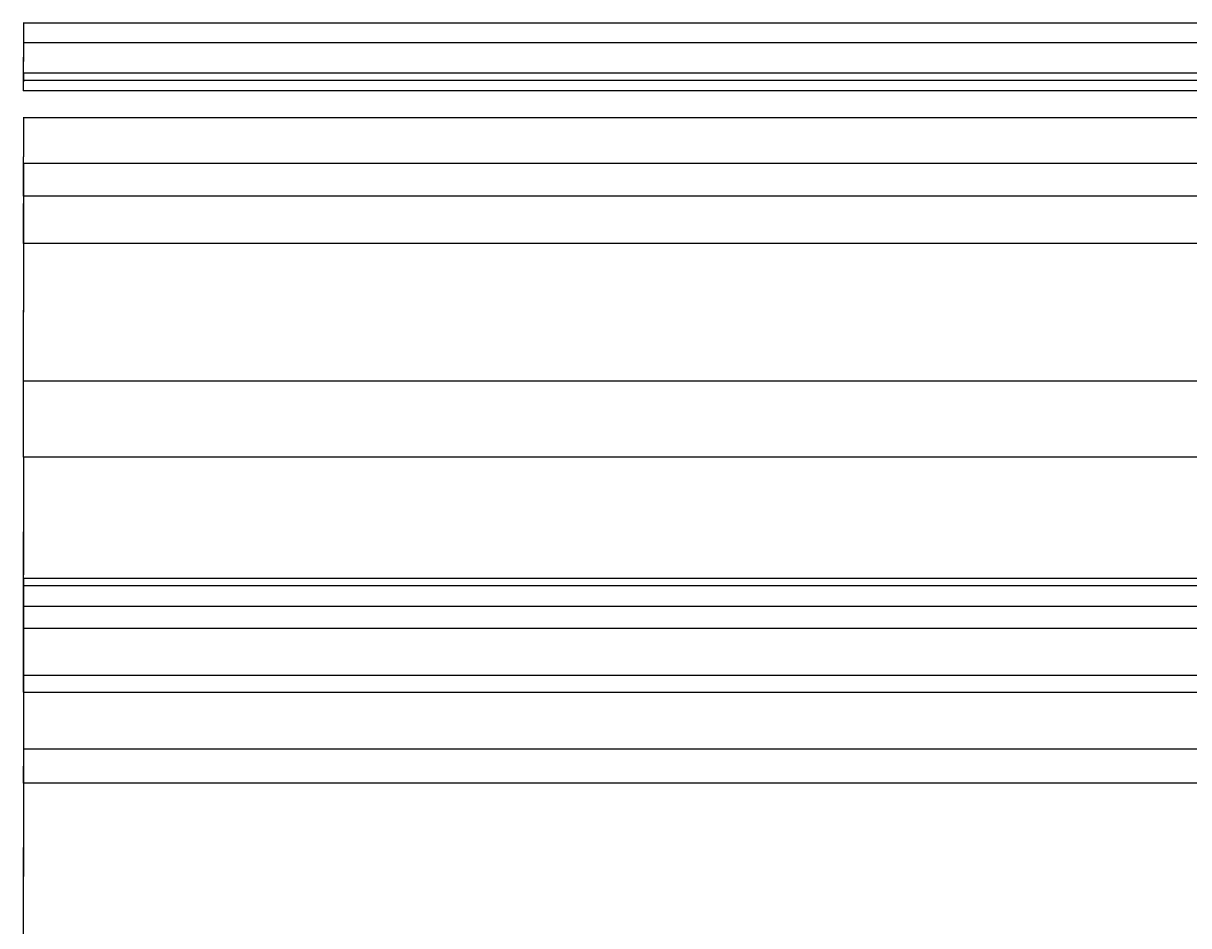
# Model space of a CAD drawing. Units: inches. Extents: x 35362 to 73946, y 43607 to 67532.
# Tile 129 of 134: x 35362 to 46600, y 56772 to 65479. Entities that reach past the tile are written whole.
import ezdxf

# ---------------------------------------------------------------- set-up
doc = ezdxf.new("R2010")
doc.units = ezdxf.units.IN
doc.header["$MEASUREMENT"] = 0
doc.layers.add('A-ANNO-DIMS', color=2, linetype='Continuous', lineweight=18)
doc.styles.get("Standard").update_dxf_attribs({"font": 'arial.ttf'})
doc.dimstyles.get("Standard").update_dxf_attribs({"dimtxt": 0.18, "dimasz": 0.18, "dimexe": 0.18, "dimexo": 0.0625, "dimgap": 0.09, "dimtad": 0, "dimtih": 1, "dimtoh": 1, "dimdec": 4, "dimzin": 0, "dimdsep": 46, "dimtxsty": 'Standard', "dimcen": 0.09, "dimadec": 0, "dimazin": 0, "dimtfac": 1, "dimtdec": 4, "dimtofl": 0, "dimtmove": 0, "dimatfit": 3, "dimfxl": 1, "dimtolj": 1, "dimtzin": 0, "dimarcsym": 0})

# ---------------------------------------------------------------- blocks, each defined once
blk = doc.blocks.new('*D12')
at = {"layer": 'A-ANNO-DIMS', "color": 0, "lineweight": -2, "transparency": 16777216}
for p, q in [((47978.60234600001, 59023.27631300003), (35361.76908500003, 59023.27631300003)), ((35361.94908500003, 59023.09631300003), (35361.94908500003, 57526.23819563782)), ((35361.94908500003, 56029.01627200003), (35361.94908500003, 57525.87438936224)), ((47978.60234600001, 56028.83627200003), (35361.76908500003, 56028.83627200003))]:
    blk.add_line(p, q, dxfattribs=at)
at = {"layer": 'A-ANNO-DIMS', "color": 0, "transparency": 16777216}
for points in [[(35361.91908500003, 59023.09631300003), (35361.97908500003, 59023.09631300003), (35361.94908500003, 59023.27631300003)], [(35361.91908500003, 56029.01627200003), (35361.97908500003, 56029.01627200003), (35361.94908500003, 56028.83627200003)]]:
    blk.add_solid(points, dxfattribs=at)
at = {"layer": 'Defpoints', "color": 0, "transparency": 16777216}
for p in [(47978.66484600001, 59023.27631300003), (35361.94908500003, 56028.83627200003), (47978.66484600001, 56028.83627200003)]:
    blk.add_point(p, dxfattribs=at)
at = {"layer": 'A-ANNO-DIMS', "color": 0, "transparency": 16777216, "insert": (35361.94908500004, 57526.05629250001), "char_height": 0.18, "attachment_point": 5}
blk.add_mtext('\\A1;2994.4', dxfattribs=at)
blk = doc.blocks.new('*D18')
at = {"layer": 'A-ANNO-DIMS', "color": 0, "lineweight": -2, "transparency": 16777216}
for p, q in [((49923.24483100003, 64127.44160800003), (35361.76908500003, 64127.44160800002)), ((35361.94908500003, 64127.26160800002), (35361.94908500003, 62710.54579452935)), ((35361.94908500003, 61293.46605200002), (35361.94908500003, 62710.18186547069)), ((49923.24483100003, 61293.28605200003), (35361.76908500003, 61293.28605200003))]:
    blk.add_line(p, q, dxfattribs=at)
at = {"layer": 'A-ANNO-DIMS', "color": 0, "transparency": 16777216}
for points in [[(35361.91908500003, 64127.26160800002), (35361.97908500003, 64127.26160800002), (35361.94908500003, 64127.44160800002)], [(35361.91908500003, 61293.46605200002), (35361.97908500003, 61293.46605200002), (35361.94908500003, 61293.28605200003)]]:
    blk.add_solid(points, dxfattribs=at)
at = {"layer": 'Defpoints', "color": 0, "transparency": 16777216}
for p in [(49923.30733100003, 64127.44160800003), (35361.94908500003, 61293.28605200003), (49923.30733100003, 61293.28605200003)]:
    blk.add_point(p, dxfattribs=at)
at = {"layer": 'A-ANNO-DIMS', "color": 0, "transparency": 16777216, "insert": (35361.94908500005, 62710.36383), "char_height": 0.18, "attachment_point": 5}
blk.add_mtext('\\A1;2834', dxfattribs=at)
blk = doc.blocks.new('*D28')
at = {"layer": 'A-ANNO-DIMS', "color": 0, "lineweight": -2, "transparency": 16777216}
for p, q in [((49923.24483100003, 61293.28605200003), (35361.76908500003, 61293.28605200003)), ((35361.94908500003, 61293.10605200002), (35361.94908500003, 60158.46308563782)), ((35361.94908500003, 59023.45631300003), (35361.94908500003, 60158.09927936224)), ((47978.60234600001, 59023.27631300003), (35361.76908500003, 59023.27631300003))]:
    blk.add_line(p, q, dxfattribs=at)
at = {"layer": 'A-ANNO-DIMS', "color": 0, "transparency": 16777216}
for points in [[(35361.91908500003, 61293.10605200002), (35361.97908500003, 61293.10605200002), (35361.94908500003, 61293.28605200003)], [(35361.91908500003, 59023.45631300003), (35361.97908500003, 59023.45631300003), (35361.94908500003, 59023.27631300003)]]:
    blk.add_solid(points, dxfattribs=at)
at = {"layer": 'Defpoints', "color": 0, "transparency": 16777216}
for p in [(49923.30733100003, 61293.28605200003), (35361.94908500003, 59023.27631300003), (47978.66484600001, 59023.27631300003)]:
    blk.add_point(p, dxfattribs=at)
at = {"layer": 'A-ANNO-DIMS', "color": 0, "transparency": 16777216, "insert": (35361.94908500005, 60158.2811825), "char_height": 0.18, "attachment_point": 5}
blk.add_mtext('\\A1;2270.0', dxfattribs=at)
blk = doc.blocks.new('*D34')
at = {"layer": 'A-ANNO-DIMS', "color": 0, "lineweight": -2, "transparency": 16777216}
for p, q in [((65335.95350800003, 61293.28605200003), (35361.76908500003, 61293.28605200003)), ((35361.94908500003, 61293.10605200002), (35361.94908500003, 60239.39690763781)), ((35361.94908500003, 59185.32395700002), (35361.94908500003, 60239.03310136224)), ((61240.84483600002, 59185.14395700003), (35361.76908500003, 59185.14395700002))]:
    blk.add_line(p, q, dxfattribs=at)
at = {"layer": 'A-ANNO-DIMS', "color": 0, "transparency": 16777216}
for points in [[(35361.91908500003, 61293.10605200002), (35361.97908500003, 61293.10605200002), (35361.94908500003, 61293.28605200003)], [(35361.91908500003, 59185.32395700002), (35361.97908500003, 59185.32395700002), (35361.94908500003, 59185.14395700002)]]:
    blk.add_solid(points, dxfattribs=at)
at = {"layer": 'Defpoints', "color": 0, "transparency": 16777216}
for p in [(65336.01600800003, 61293.28605200003), (35361.94908500003, 59185.14395700002), (61240.90733600002, 59185.14395700003)]:
    blk.add_point(p, dxfattribs=at)
at = {"layer": 'A-ANNO-DIMS', "color": 0, "transparency": 16777216, "insert": (35361.94908500005, 60239.2150045), "char_height": 0.18, "attachment_point": 5}
blk.add_mtext('\\A1;2108.1', dxfattribs=at)
blk = doc.blocks.new('*D36')
at = {"layer": 'A-ANNO-DIMS', "color": 0, "lineweight": -2, "transparency": 16777216}
for p, q in [((68320.80826200004, 60122.34633200002), (35361.76908500003, 60122.34633200002)), ((35361.94908500003, 60122.16633200002), (35361.94908500003, 57247.82893113781)), ((35361.94908500003, 54373.12772400002), (35361.94908500003, 57247.46512486223)), ((68320.80826200004, 54372.94772400003), (35361.76908500003, 54372.94772400002))]:
    blk.add_line(p, q, dxfattribs=at)
at = {"layer": 'A-ANNO-DIMS', "color": 0, "transparency": 16777216}
for points in [[(35361.91908500003, 60122.16633200002), (35361.97908500003, 60122.16633200002), (35361.94908500003, 60122.34633200002)], [(35361.91908500003, 54373.12772400002), (35361.97908500003, 54373.12772400002), (35361.94908500003, 54372.94772400002)]]:
    blk.add_solid(points, dxfattribs=at)
at = {"layer": 'Defpoints', "color": 0, "transparency": 16777216}
for p in [(68320.87076200004, 60122.34633200002), (35361.94908500003, 54372.94772400002), (68320.87076200004, 54372.94772400003)]:
    blk.add_point(p, dxfattribs=at)
at = {"layer": 'A-ANNO-DIMS', "color": 0, "transparency": 16777216, "insert": (35361.94908500004, 57247.64702799999), "char_height": 0.18, "attachment_point": 5}
blk.add_mtext('\\A1;5749.4', dxfattribs=at)
blk = doc.blocks.new('*D45')
at = {"layer": 'A-ANNO-DIMS', "color": 0, "lineweight": -2, "transparency": 16777216}
for p, q in [((52517.73527400002, 65478.87035600003), (35361.76908500003, 65478.87035600002)), ((35361.94908500003, 65478.69035600002), (35361.94908500003, 65153.89527602935)), ((35361.94908500003, 64828.73626700002), (35361.94908500003, 65153.53134697069)), ((52517.73527400002, 64828.55626700002), (35361.76908500003, 64828.55626700002))]:
    blk.add_line(p, q, dxfattribs=at)
at = {"layer": 'A-ANNO-DIMS', "color": 0, "transparency": 16777216}
for points in [[(35361.91908500003, 65478.69035600002), (35361.97908500003, 65478.69035600002), (35361.94908500003, 65478.87035600002)], [(35361.91908500003, 64828.73626700002), (35361.97908500003, 64828.73626700002), (35361.94908500003, 64828.55626700002)]]:
    blk.add_solid(points, dxfattribs=at)
at = {"layer": 'Defpoints', "color": 0, "transparency": 16777216}
for p in [(52517.79777400003, 65478.87035600003), (35361.94908500003, 64828.55626700002), (52517.79777400003, 64828.55626700002)]:
    blk.add_point(p, dxfattribs=at)
at = {"layer": 'A-ANNO-DIMS', "color": 0, "transparency": 16777216, "insert": (35361.94908500005, 65153.7133115), "char_height": 0.18, "attachment_point": 5}
blk.add_mtext('\\A1;650.3', dxfattribs=at)
blk = doc.blocks.new('*D48')
at = {"layer": 'A-ANNO-DIMS', "color": 0, "lineweight": -2, "transparency": 16777216}
for p, q in [((56457.22713600003, 58474.86812300003), (35361.76908500003, 58474.86812300002)), ((35361.94908500003, 58474.68812300002), (35361.94908500003, 58311.09546902935)), ((35361.94908500003, 58147.13888600002), (35361.94908500003, 58310.73153997069)), ((56457.22713600003, 58146.95888600002), (35361.76908500003, 58146.95888600002))]:
    blk.add_line(p, q, dxfattribs=at)
at = {"layer": 'A-ANNO-DIMS', "color": 0, "transparency": 16777216}
for points in [[(35361.91908500003, 58474.68812300002), (35361.97908500003, 58474.68812300002), (35361.94908500003, 58474.86812300002)], [(35361.91908500003, 58147.13888600002), (35361.97908500003, 58147.13888600002), (35361.94908500003, 58146.95888600002)]]:
    blk.add_solid(points, dxfattribs=at)
at = {"layer": 'Defpoints', "color": 0, "transparency": 16777216}
for p in [(56457.28963600003, 58474.86812300003), (35361.94908500003, 58146.95888600002), (56457.28963600003, 58146.95888600002)]:
    blk.add_point(p, dxfattribs=at)
at = {"layer": 'A-ANNO-DIMS', "color": 0, "transparency": 16777216, "insert": (35361.94908500004, 58310.9135045), "char_height": 0.18, "attachment_point": 5}
blk.add_mtext('\\A1;327.9', dxfattribs=at)
blk = doc.blocks.new('*D73')
at = {"layer": 'A-ANNO-DIMS', "color": 0, "lineweight": -2, "transparency": 16777216}
for p, q in [((59468.73309100003, 64567.97198600003), (35361.76908500003, 64567.97198600002)), ((35361.94908500003, 64567.79198600002), (35361.94908500003, 64189.84474213781)), ((35361.94908500003, 63811.53369200002), (35361.94908500003, 64189.48093586223)), ((59468.73309100003, 63811.35369200002), (35361.76908500003, 63811.35369200002))]:
    blk.add_line(p, q, dxfattribs=at)
at = {"layer": 'A-ANNO-DIMS', "color": 0, "transparency": 16777216}
for points in [[(35361.91908500003, 64567.79198600002), (35361.97908500003, 64567.79198600002), (35361.94908500003, 64567.97198600002)], [(35361.91908500003, 63811.53369200002), (35361.97908500003, 63811.53369200002), (35361.94908500003, 63811.35369200002)]]:
    blk.add_solid(points, dxfattribs=at)
at = {"layer": 'Defpoints', "color": 0, "transparency": 16777216}
for p in [(35361.94908500003, 64567.97198600002), (59468.79559100003, 64567.97198600003), (59468.79559100003, 63811.35369200002)]:
    blk.add_point(p, dxfattribs=at)
at = {"layer": 'A-ANNO-DIMS', "color": 0, "transparency": 16777216, "insert": (35361.94908500005, 64189.66283899999), "char_height": 0.18, "attachment_point": 5}
blk.add_mtext('\\A1;756.6', dxfattribs=at)
blk = doc.blocks.new('*D93')
at = {"layer": 'A-ANNO-DIMS', "color": 0, "lineweight": -2, "transparency": 16777216}
for p, q in [((50377.69713900003, 63354.17630000002), (35361.76908500003, 63354.17630000002)), ((35361.94908500003, 63353.99630000002), (35361.94908500003, 62690.28238902935)), ((35361.94908500003, 62026.20454900002), (35361.94908500003, 62689.91845997069)), ((50377.69713900003, 62026.02454900003), (35361.76908500003, 62026.02454900002))]:
    blk.add_line(p, q, dxfattribs=at)
at = {"layer": 'A-ANNO-DIMS', "color": 0, "transparency": 16777216}
for points in [[(35361.91908500003, 63353.99630000002), (35361.97908500003, 63353.99630000002), (35361.94908500003, 63354.17630000002)], [(35361.91908500003, 62026.20454900002), (35361.97908500003, 62026.20454900002), (35361.94908500003, 62026.02454900002)]]:
    blk.add_solid(points, dxfattribs=at)
at = {"layer": 'Defpoints', "color": 0, "transparency": 16777216}
for p in [(50377.75963900003, 63354.17630000002), (35361.94908500003, 62026.02454900002), (50377.75963900003, 62026.02454900003)]:
    blk.add_point(p, dxfattribs=at)
at = {"layer": 'A-ANNO-DIMS', "color": 0, "transparency": 16777216, "insert": (35361.94908500005, 62690.1004245), "char_height": 0.18, "attachment_point": 5}
blk.add_mtext('\\A1;1328.2', dxfattribs=at)
blk = doc.blocks.new('*D95')
at = {"layer": 'A-ANNO-DIMS', "color": 0, "lineweight": -2, "transparency": 16777216}
for p, q in [((49923.24483100003, 64127.44160800003), (35361.76908500003, 64127.44160800002)), ((35361.94908500003, 64127.26160800002), (35361.94908500003, 63740.99091852935)), ((35361.94908500003, 63354.35630000002), (35361.94908500003, 63740.62698947069)), ((50377.69713900003, 63354.17630000002), (35361.76908500003, 63354.17630000002))]:
    blk.add_line(p, q, dxfattribs=at)
at = {"layer": 'A-ANNO-DIMS', "color": 0, "transparency": 16777216}
for points in [[(35361.91908500003, 64127.26160800002), (35361.97908500003, 64127.26160800002), (35361.94908500003, 64127.44160800002)], [(35361.91908500003, 63354.35630000002), (35361.97908500003, 63354.35630000002), (35361.94908500003, 63354.17630000002)]]:
    blk.add_solid(points, dxfattribs=at)
at = {"layer": 'Defpoints', "color": 0, "transparency": 16777216}
for p in [(49923.30733100003, 64127.44160800003), (35361.94908500003, 63354.17630000002), (50377.75963900003, 63354.17630000002)]:
    blk.add_point(p, dxfattribs=at)
at = {"layer": 'A-ANNO-DIMS', "color": 0, "transparency": 16777216, "insert": (35361.94908500005, 63740.808954), "char_height": 0.18, "attachment_point": 5}
blk.add_mtext('\\A1;773.3', dxfattribs=at)
blk = doc.blocks.new('*D98')
at = {"layer": 'A-ANNO-DIMS', "color": 0, "lineweight": -2, "transparency": 16777216}
for p, q in [((53366.70323300003, 64997.68268100003), (35361.76908500003, 64997.68268100002)), ((35361.94908500003, 64997.50268100002), (35361.94908500003, 64913.30143852935)), ((35361.94908500003, 64828.73626700002), (35361.94908500003, 64912.93750947069)), ((52517.73527400002, 64828.55626700002), (35361.76908500003, 64828.55626700002))]:
    blk.add_line(p, q, dxfattribs=at)
at = {"layer": 'A-ANNO-DIMS', "color": 0, "transparency": 16777216}
for points in [[(35361.91908500003, 64997.50268100002), (35361.97908500003, 64997.50268100002), (35361.94908500003, 64997.68268100002)], [(35361.91908500003, 64828.73626700002), (35361.97908500003, 64828.73626700002), (35361.94908500003, 64828.55626700002)]]:
    blk.add_solid(points, dxfattribs=at)
at = {"layer": 'Defpoints', "color": 0, "transparency": 16777216}
for p in [(53366.76573300002, 64997.68268100003), (35361.94908500003, 64828.55626700002), (52517.79777400003, 64828.55626700002)]:
    blk.add_point(p, dxfattribs=at)
at = {"layer": 'A-ANNO-DIMS', "color": 0, "transparency": 16777216, "insert": (35361.94908500005, 64913.11947399999), "char_height": 0.18, "attachment_point": 5}
blk.add_mtext('\\A1;169.13', dxfattribs=at)
blk = doc.blocks.new('*D101')
at = {"layer": 'A-ANNO-DIMS', "color": 0, "lineweight": -2, "transparency": 16777216}
for p, q in [((52897.41774600003, 65291.58881700003), (35361.76908500003, 65291.58881700002)), ((35361.94908500003, 65291.40881700002), (35361.94908500003, 65109.04535402935)), ((35361.94908500003, 64926.31796200002), (35361.94908500003, 65108.68142497069)), ((53150.59930100002, 64926.13796200003), (35361.76908500003, 64926.13796200002))]:
    blk.add_line(p, q, dxfattribs=at)
at = {"layer": 'A-ANNO-DIMS', "color": 0, "transparency": 16777216}
for points in [[(35361.91908500003, 65291.40881700002), (35361.97908500003, 65291.40881700002), (35361.94908500003, 65291.58881700002)], [(35361.91908500003, 64926.31796200002), (35361.97908500003, 64926.31796200002), (35361.94908500003, 64926.13796200002)]]:
    blk.add_solid(points, dxfattribs=at)
at = {"layer": 'Defpoints', "color": 0, "transparency": 16777216}
for p in [(52897.48024600003, 65291.58881700003), (35361.94908500003, 64926.13796200002), (53150.66180100003, 64926.13796200003)]:
    blk.add_point(p, dxfattribs=at)
at = {"layer": 'A-ANNO-DIMS', "color": 0, "transparency": 16777216, "insert": (35361.94908500005, 65108.8633895), "char_height": 0.18, "attachment_point": 5}
blk.add_mtext('\\A1;365.45', dxfattribs=at)
blk = doc.blocks.new('*D108')
at = {"layer": 'A-ANNO-DIMS', "color": 0, "lineweight": -2, "transparency": 16777216}
for p, q in [((50259.66194000003, 60051.66084400003), (35361.76908500003, 60051.66084400002)), ((35361.94908500003, 60051.48084400002), (35361.94908500003, 59845.07863052935)), ((35361.94908500003, 59638.31248800002), (35361.94908500003, 59844.71470147069)), ((50483.03225800003, 59638.13248800003), (35361.76908500003, 59638.13248800002))]:
    blk.add_line(p, q, dxfattribs=at)
at = {"layer": 'A-ANNO-DIMS', "color": 0, "transparency": 16777216}
for points in [[(35361.91908500003, 60051.48084400002), (35361.97908500003, 60051.48084400002), (35361.94908500003, 60051.66084400002)], [(35361.91908500003, 59638.31248800002), (35361.97908500003, 59638.31248800002), (35361.94908500003, 59638.13248800002)]]:
    blk.add_solid(points, dxfattribs=at)
at = {"layer": 'Defpoints', "color": 0, "transparency": 16777216}
for p in [(50259.72444000003, 60051.66084400003), (35361.94908500003, 59638.13248800002), (50483.09475800002, 59638.13248800003)]:
    blk.add_point(p, dxfattribs=at)
at = {"layer": 'A-ANNO-DIMS', "color": 0, "transparency": 16777216, "insert": (35361.94908500005, 59844.896666), "char_height": 0.18, "attachment_point": 5}
blk.add_mtext('\\A1;413.5', dxfattribs=at)
blk = doc.blocks.new('*D110')
at = {"layer": 'A-ANNO-DIMS', "color": 0, "lineweight": -2, "transparency": 16777216}
for p, q in [((49923.24483100003, 61293.28605200003), (35361.76908500003, 61293.28605200003)), ((35361.94908500003, 61293.10605200002), (35361.94908500003, 60571.86342902935)), ((35361.94908500003, 59850.25687700002), (35361.94908500003, 60571.49949997069)), ((50139.50021400003, 59850.07687700003), (35361.76908500003, 59850.07687700002))]:
    blk.add_line(p, q, dxfattribs=at)
at = {"layer": 'A-ANNO-DIMS', "color": 0, "transparency": 16777216}
for points in [[(35361.91908500003, 61293.10605200002), (35361.97908500003, 61293.10605200002), (35361.94908500003, 61293.28605200003)], [(35361.91908500003, 59850.25687700002), (35361.97908500003, 59850.25687700002), (35361.94908500003, 59850.07687700002)]]:
    blk.add_solid(points, dxfattribs=at)
at = {"layer": 'Defpoints', "color": 0, "transparency": 16777216}
for p in [(49923.30733100003, 61293.28605200003), (35361.94908500003, 59850.07687700002), (50139.56271400003, 59850.07687700003)]:
    blk.add_point(p, dxfattribs=at)
at = {"layer": 'A-ANNO-DIMS', "color": 0, "transparency": 16777216, "insert": (35361.94908500005, 60571.6814645), "char_height": 0.18, "attachment_point": 5}
blk.add_mtext('\\A1;1443.2', dxfattribs=at)

msp = doc.modelspace()

# ---------------------------------------------------------------- dimensions: what is measured, and where the dimension line sits
at = {"layer": 'A-ANNO-DIMS'}
for base, p1, p2, override, picture, middle in [((35361.94908500003, 64828.55626700002), (52517.797774, 65478.870356), (52517.797774, 64828.556267), {"dimdec": 1, "dimlfac": 1, "dimrnd": 0, "dimzin": 0, "dimdsep": 46, "dimlunit": 2}, '*D45', (35361.94908500005, 65153.7133115)), ((35361.94908500003, 64926.13796200002), (52897.480246, 65291.588817), (53150.661801, 64926.137962), {"dimdec": 2, "dimlfac": 1, "dimrnd": 0, "dimzin": 0, "dimdsep": 46, "dimlunit": 2}, '*D101', (35361.94908500005, 65108.8633895)), ((35361.94908500003, 64828.55626700002), (53366.765733, 64997.682681), (52517.797774, 64828.556267), {"dimdec": 2, "dimlfac": 1, "dimrnd": 0, "dimzin": 0, "dimdsep": 46, "dimlunit": 2}, '*D98', (35361.94908500005, 64913.11947399999)), ((35361.94908500003, 64567.97198600002), (59468.795591, 63811.35369199999), (59468.795591, 64567.971986), {"dimdec": 1, "dimlfac": 1, "dimrnd": 0, "dimzin": 0, "dimdsep": 46, "dimlunit": 2}, '*D73', (35361.94908500005, 64189.66283899999)), ((35361.94908500003, 63354.17630000002), (49923.307331, 64127.44160799999), (50377.759639, 63354.1763), {"dimdec": 1, "dimlfac": 1, "dimrnd": 0, "dimzin": 0, "dimdsep": 46, "dimlunit": 2}, '*D95', (35361.94908500005, 63740.808954)), ((35361.94908500003, 61293.28605200003), (49923.307331, 64127.44160799999), (49923.307331, 61293.286052), {"dimdec": 0, "dimlfac": 1, "dimrnd": 0, "dimzin": 0, "dimdsep": 46, "dimlunit": 2}, '*D18', (35361.94908500005, 62710.36383)), ((35361.94908500003, 62026.02454900002), (50377.759639, 63354.1763), (50377.759639, 62026.024549), {"dimdec": 1, "dimlfac": 1, "dimrnd": 0, "dimzin": 0, "dimdsep": 46, "dimlunit": 2}, '*D93', (35361.94908500005, 62690.1004245)), ((35361.94908500003, 59023.27631300003), (49923.307331, 61293.286052), (47978.664846, 59023.276313), {"dimdec": 1, "dimlfac": 1, "dimrnd": 0, "dimzin": 0, "dimdsep": 46, "dimlunit": 2}, '*D28', (35361.94908500005, 60158.2811825)), ((35361.94908500003, 59185.14395700002), (65336.01600799999, 61293.286052), (61240.907336, 59185.14395699999), {"dimdec": 1, "dimlfac": 1, "dimrnd": 0, "dimzin": 0, "dimdsep": 46, "dimlunit": 2}, '*D34', (35361.94908500005, 60239.2150045)), ((35361.94908500003, 59850.07687700002), (49923.307331, 61293.286052), (50139.562714, 59850.076877), {"dimdec": 1, "dimlfac": 1, "dimrnd": 0, "dimzin": 0, "dimdsep": 46, "dimlunit": 2}, '*D110', (35361.94908500005, 60571.6814645)), ((35361.94908500003, 54372.94772400002), (68320.870762, 60122.346332), (68320.870762, 54372.947724), {"dimdec": 1, "dimlfac": 1, "dimrnd": 0, "dimzin": 0, "dimdsep": 46, "dimlunit": 2}, '*D36', (35361.94908500004, 57247.64702799999)), ((35361.94908500003, 59638.13248800002), (50259.72443999999, 60051.66084399999), (50483.094758, 59638.132488), {"dimdec": 1, "dimlfac": 1, "dimrnd": 0, "dimzin": 0, "dimdsep": 46, "dimlunit": 2}, '*D108', (35361.94908500005, 59844.896666)), ((35361.94908500003, 56028.83627200003), (47978.664846, 59023.276313), (47978.664846, 56028.836272), {"dimdec": 1, "dimlfac": 1, "dimrnd": 0, "dimzin": 0, "dimdsep": 46, "dimlunit": 2}, '*D12', (35361.94908500004, 57526.05629250001)), ((35361.94908500003, 58146.95888600002), (56457.289636, 58474.868123), (56457.289636, 58146.958886), {"dimdec": 1, "dimlfac": 1, "dimrnd": 0, "dimzin": 0, "dimdsep": 46, "dimlunit": 2}, '*D48', (35361.94908500004, 58310.9135045))]:
    dim = msp.add_linear_dim(base=base, p1=p1, p2=p2, angle=90, dimstyle='Standard', override=override, dxfattribs=at)
    dim.commit()
    dim.dimension.update_dxf_attribs({"geometry": picture, "text_midpoint": middle})

doc.saveas('drawing.dxf')
